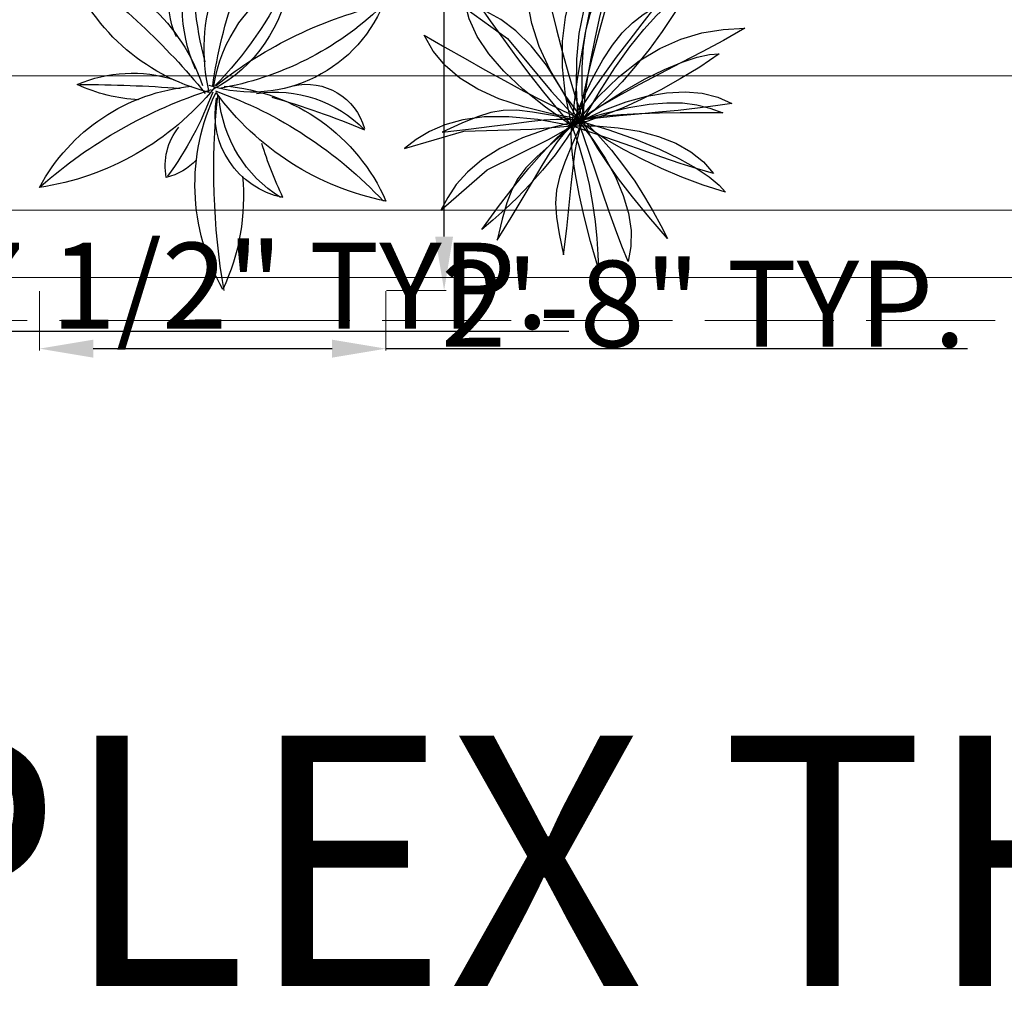
# Model space of a CAD drawing. Units: inches. Extents: x 351 to 1738, y -265 to 286.
# Tile 15 of 38: x 1176 to 1268, y -265 to -175. Entities that reach past the tile are written whole.
import ezdxf

# ---------------------------------------------------------------- set-up
doc = ezdxf.new("R2010")
doc.units = ezdxf.units.IN
doc.header["$MEASUREMENT"] = 0
doc.linetypes.add('ACAD_ISO02W100', pattern=[15, 12, -3])
for name, color, linetype, lineweight in [('A-ANNO-DIMS', 2, 'Continuous', 18), ('A-ANNO-TITL', 7, 'Continuous', 35), ('A-FLOR-OVHD', 1, 'ACAD_ISO02W100', 18), ('A-FLOR-PATT', 9, 'Continuous', 9)]:
    doc.layers.add(name, color=color, linetype=linetype, lineweight=lineweight)
for name, color, linetype in [('CAY', 94, 'Continuous'), ('CHITIET', 144, 'Continuous'), ('DIENHOA', 3, 'Continuous'), ('netmanh', 9, 'Continuous'), ('VATDUNG', 9, 'Continuous')]:
    doc.layers.add(name, color=color, linetype=linetype)
doc.styles.add('Annotative', font='arial.ttf')
doc.styles.get("Standard").update_dxf_attribs({"font": 'arial.ttf'})
doc.dimstyles.get("Standard").update_dxf_attribs({"dimtxt": 8, "dimasz": 5, "dimexe": 0.18, "dimexo": 0.0625, "dimgap": 0.09, "dimtad": 1, "dimtoh": 1, "dimzin": 0, "dimdsep": 46, "dimlunit": 4, "dimtxsty": 'Standard', "dimcen": 0, "dimclre": 256, "dimadec": 0, "dimazin": 0, "dimtfac": 1, "dimtofl": 0, "dimtmove": 0, "dimatfit": 3, "dimfxl": 1, "dimtolj": 1, "dimtzin": 0, "dimlwe": -1, "dimarcsym": 0})

# ---------------------------------------------------------------- blocks, each defined once
blk = doc.blocks.new('Cay03_mb')
at = {"layer": 'DIENHOA'}
for p, q in [((118.6, 555.3), (166.2, 599.1)), ((166.2, 599.1), (142.2, 519.4)), ((79.5, 503.7), (118.6, 555.3)), ((142.2, 519.4), (119, 441.7)), ((48.6, 443.6), (79.5, 503.7)), ((25.5, 374.3), (48.6, 443.6)), ((119, 441.7), (96.7, 365.6)), ((-365.2, 390.3), (-414.4, 402.8)), ((-414.4, 402.8), (-240.2, 277.8)), ((-314.9, 371.3), (-365.2, 390.3)), ((-263.5, 343.5), (-314.9, 371.3)), ((-211.2, 304.6), (-263.5, 343.5)), ((9.9, 295.3), (25.5, 374.3)), ((96.7, 365.6), (75.6, 290.6)), ((436.8, 297.2), (511, 309.6)), ((511, 309.6), (585.9, 313.5)), ((585.9, 313.5), (511.8, 271.4)), ((-240.2, 277.8), (-88.4, 94.9)), ((-158, 252.3), (-211.2, 304.6)), ((1.6, 205.7), (9.9, 295.3)), ((75.6, 290.6), (55.7, 216.3)), ((290.6, 243.2), (363.4, 275.4)), ((363.4, 275.4), (436.8, 297.2)), ((-104.2, 184.4), (-158, 252.3)), ((218.5, 199.8), (290.6, 243.2)), ((511.8, 271.4), (437.6, 231.5)), ((55.7, 216.3), (37.3, 142.1)), ((437.6, 231.5), (363.7, 192.9)), ((-49.6, 98.5), (-104.2, 184.4)), ((0.2, 104.9), (1.6, 205.7)), ((147, 144.1), (218.5, 199.8)), ((363.7, 192.9), (290.2, 154.9)), ((37.3, 142.1), (20.5, 67.6)), ((75.9, 75.2), (147, 144.1)), ((290.2, 154.9), (217.4, 116.6)), ((5.4, -7.8), (0.2, 104.9)), ((217.4, 116.6), (145.5, 77.3)), ((-88.4, 94.9), (5.4, -7.8)), ((5.4, -7.8), (-49.6, 98.5)), ((5.4, -7.8), (75.9, 75.2)), ((145.5, 77.3), (74.7, 36.1)), ((20.5, 67.6), (5.4, -7.8)), ((74.7, 36.1), (5.4, -7.8)), ((100.3, 18.4), (182.2, 37.2)), ((182.2, 37.2), (253, 48.9)), ((253, 48.9), (314.6, 54.1)), ((314.6, 54.1), (369.2, 53.3)), ((369.2, 53.3), (418.6, 46.8)), ((418.6, 46.8), (464.9, 35.2)), ((464.9, 35.2), (510, 19)), ((-345, 5.4), (-399.6, -17.1)), ((-298.6, 20.1), (-345, 5.4)), ((-254.7, 27.4), (-298.6, 20.1)), ((-208, 27.8), (-254.7, 27.4)), ((-152.7, 21.7), (-208, 27.8)), ((-83.4, 9.7), (-152.7, 21.7)), ((5.4, -7.8), (-83.4, 9.7)), ((5.4, -7.8), (100.3, 18.4)), ((46.3, 0.9), (5.4, -7.8)), ((96.7, 7.5), (46.3, 0.9)), ((155, 12.2), (96.7, 7.5)), ((219.6, 15.4), (155, 12.2)), ((289, 17.4), (219.6, 15.4)), ((361.6, 18.5), (289, 17.4)), ((435.8, 18.9), (361.6, 18.5)), ((510, 19), (435.8, 18.9)), ((-399.6, -17.1), (-468, -47.9)), ((-375.6, -37.8), (-295.3, -27.9)), ((-295.3, -27.9), (-225.8, -18.9)), ((-225.8, -18.9), (-165.8, -11.3)), ((-165.8, -11.3), (-114, -5.7)), ((-114, -5.7), (-69, -2.9)), ((-69, -2.9), (-29.6, -3.4)), ((-45.1, -46.3), (-16.5, -22.4)), ((5.4, -7.8), (-33.2, -69.5)), ((-29.6, -3.4), (5.4, -7.8)), ((-16.5, -22.4), (5.4, -7.8)), ((5.4, -7.8), (56.8, -73.3)), ((25.9, -64.4), (5.4, -7.8)), ((5.4, -7.8), (112.8, -40.3)), ((53.5, -41.6), (5.4, -7.8)), ((-468, -47.9), (-375.6, -37.8)), ((-79.8, -79.6), (-45.1, -46.3)), ((47, -125.9), (25.9, -64.4)), ((107, -75.7), (53.5, -41.6)), ((112.8, -40.3), (207.5, -73.8)), ((-120.2, -122.1), (-79.8, -79.6)), ((-33.2, -69.5), (-74.6, -127.3)), ((56.8, -73.3), (100.4, -139.1)), ((165.5, -109.6), (107, -75.7)), ((207.5, -73.8), (289.5, -107.6)), ((-165.9, -174.1), (-120.2, -122.1)), ((-74.6, -127.3), (-117.8, -181.1)), ((68.7, -190.6), (47, -125.9)), ((228.7, -142.8), (165.5, -109.6)), ((289.5, -107.6), (359.3, -141.1)), ((100.4, -139.1), (135.9, -204.3)), ((296, -174.7), (228.7, -142.8)), ((359.3, -141.1), (416.9, -173.5)), ((-216.3, -235.6), (-165.9, -174.1)), ((-117.8, -181.1), (-162.1, -230.9)), ((90.8, -256.6), (68.7, -190.6)), ((135.9, -204.3), (162.8, -268.3)), ((367.1, -204.8), (296, -174.7)), ((441.6, -232.7), (367.1, -204.8)), ((416.9, -173.5), (462.6, -204.2)), ((462.6, -204.2), (496.5, -232.5)), ((-271, -306.6), (-216.3, -235.6)), ((-162.1, -230.9), (-206.3, -276.5)), ((518.9, -257.7), (441.6, -232.7)), ((496.5, -232.5), (518.9, -257.7)), ((113.1, -322.2), (90.8, -256.6)), ((162.8, -268.3), (181, -330.4)), ((-329.5, -387.1), (-271, -306.6)), ((-206.3, -276.5), (-249.6, -317.8)), ((-249.6, -317.8), (-291, -354.7)), ((135.4, -385.6), (113.1, -322.2)), ((181, -330.4), (190, -390)), ((-291, -354.7), (-329.5, -387.1)), ((157.6, -445), (135.4, -385.6)), ((190, -390), (189.6, -446.3)), ((179.5, -498.7), (157.6, -445)), ((189.6, -446.3), (179.5, -498.7))]:
    blk.add_line(p, q, dxfattribs=at)
for points in [[(23.7, -5.4), (-41, 82.2), (-91.8, 167.1), (-129.7, 249.5), (-155.6, 329.6), (-170.2, 407.8), (-174.7, 484.2), (-169.8, 559.3), (-156.5, 633.1)], [(-156.5, 633.1), (-132.5, 551.3), (-110.5, 470), (-89.8, 389.2), (-69.6, 309), (-49, 229.4), (-27.1, 150.4), (-3.2, 72.1), (23.7, -5.4)], [(-16.4, -26.7), (-38.3, 80), (-48.9, 178.3), (-48.7, 269), (-38.5, 352.6), (-19.1, 429.7), (9, 501), (44.9, 567.1), (87.9, 628.5)], [(87.9, 628.5), (75.5, 544.2), (61.3, 461.2), (46.1, 379.1), (30.8, 297.8), (16.1, 216.9), (2.9, 136), (-8.3, 54.9), (-16.4, -26.7)], [(23.7, -5.4), (19.8, 93), (20.3, 177), (25, 248.5), (34, 309.8), (47.3, 362.7), (64.9, 409.3), (86.8, 451.7), (112.9, 491.9)], [(112.9, 491.9), (96, 419.7), (79.5, 347.4), (63.9, 276.5), (50, 208.4), (38.4, 144.8), (29.7, 86.9), (24.6, 36.3), (23.7, -5.4)], [(-395.6, 473.7), (-347.5, 405.6), (-300.6, 339.5), (-254.3, 275.1), (-208.3, 212.3), (-161.9, 150.9), (-114.8, 90.7), (-66.5, 31.6), (-16.4, -26.7)], [(-16.4, -26.7), (-108.3, 38.6), (-186.9, 101.7), (-252.4, 163.5), (-305.1, 224.4), (-345.4, 285.2), (-373.7, 346.6), (-390.4, 409.2), (-395.6, 473.7)], [(384.3, 437.5), (342.2, 367.8), (298.1, 301.7), (252.6, 239.4), (206.1, 181.1), (159.4, 127.2), (113, 78), (67.6, 33.6), (23.7, -5.4)], [(23.7, -5.4), (79.9, 91.7), (134.1, 176.2), (185.8, 248.4), (234.3, 308.7), (279, 357.3), (319.3, 394.8), (354.6, 421.4), (384.3, 437.5)], [(273.2, 387.3), (227.6, 328.8), (182.3, 270.1), (138.4, 212.3), (97.2, 156.4), (60, 103.4), (27.8, 54.6), (1.9, 10.8), (-16.4, -26.7)], [(-16.4, -26.7), (21.4, 64.2), (57, 140.3), (91.4, 203.3), (125.2, 255.1), (159.5, 297.5), (195, 332.5), (232.7, 361.8), (273.2, 387.3)], [(-530.5, 289.7), (-458.3, 248.1), (-387.9, 207.8), (-318.9, 168.7), (-250.8, 131.1), (-182.9, 94.8), (-114.9, 59.9), (-46.2, 26.5), (23.7, -5.4)], [(23.7, -5.4), (-87.2, 15.2), (-185, 39.6), (-270.3, 68.2), (-343.7, 101.4), (-405.9, 139.7), (-457.3, 183.5), (-498.7, 233.4), (-530.5, 289.7)], [(496.7, 224), (429.4, 178.4), (361.6, 136.9), (294.1, 99.5), (227.5, 66.1), (162.4, 36.7), (99.7, 11.5), (39.8, -9.7), (-16.4, -26.7)], [(-16.4, -26.7), (75.4, 37.9), (160.1, 91.8), (237.3, 135.7), (306.6, 170), (367.6, 195.4), (419.9, 212.5), (463.1, 221.9), (496.7, 224)], [(23.7, -5.4), (99.3, 29.7), (173.2, 57.1), (244.8, 76.7), (313.3, 88.3), (377.9, 91.8), (437.9, 87), (492.7, 73.8), (541.4, 52)], [(541.4, 52), (484.1, 42.9), (421.2, 34.8), (354.4, 27.6), (285.4, 20.9), (216.1, 14.5), (148.2, 8.1), (83.5, 1.6), (23.7, -5.4)], [(-16.4, -26.7), (-134, -4.7), (-235.3, 5.3), (-322, 4.7), (-395.9, -5), (-458.7, -22.3), (-512.3, -45.7), (-558.2, -73.6), (-598.4, -104.7)], [(-598.4, -104.7), (-392.7, -44.4), (-155, -37.4), (-16.4, -26.7)], [(-471.9, -320.3), (-310.5, -179.3), (-97.7, -73.3), (23.7, -5.4)], [(23.7, -5.4), (-92.3, -34.8), (-188.4, -68.2), (-266.9, -105.1), (-329.9, -144.9), (-379.7, -187), (-418.5, -230.7), (-448.5, -275.3), (-471.9, -320.3)], [(-276.2, -424.4), (-227.3, -345.4), (-185.7, -276.1), (-150, -215.7), (-119.1, -163.8), (-91.5, -119.5), (-66, -82.3), (-41.4, -51.6), (-16.4, -26.7)], [(-16.4, -26.7), (-84.9, -86), (-137, -133.1), (-175.8, -173), (-204.3, -210), (-225.5, -249.1), (-242.5, -294.7), (-258.4, -351.6), (-276.2, -424.4)], [(23.7, -5.4), (-13.6, -87.9), (-41.1, -152.6), (-59.6, -205), (-69.9, -250.7), (-72.8, -295), (-69.2, -343.6), (-59.7, -401.9), (-45.3, -475.5)], [(-45.3, -475.5), (-34.1, -383.2), (-25.4, -302.8), (-18.3, -233.1), (-12, -172.9), (-5.6, -121.2), (2, -76.8), (11.4, -38.5), (23.7, -5.4)], [(76.2, -524.2), (48.8, -428.5), (26.6, -341.7), (9.2, -264.1), (-3.6, -196.1), (-12.3, -138), (-17.1, -90.2), (-18.3, -53), (-16.4, -26.7)], [(-16.4, -26.7), (66.9, -26.6), (145.6, -32.7), (218.8, -44.9), (285.8, -63.1), (345.9, -87.1), (398.4, -116.6), (442.6, -151.6), (477.6, -191.8)], [(477.6, -191.8), (421.8, -176), (361.3, -156.9), (297.6, -135.5), (232.2, -112.6), (166.6, -89.4), (102.3, -66.6), (40.8, -45.4), (-16.4, -26.7)], [(-16.4, -26.7), (8.5, -95.1), (28.5, -163.3), (44.3, -230.6), (56.3, -296.1), (65, -359), (70.9, -418.5), (74.5, -473.9), (76.2, -524.2)], [(316.5, -418.1), (251.4, -342.8), (194.8, -273.3), (146.5, -210.2), (106.3, -153.8), (74.1, -104.7), (49.7, -63.4), (32.9, -30.1), (23.7, -5.4)], [(23.7, -5.4), (74.9, -57.1), (121.8, -110.6), (164.3, -165), (202.7, -219.4), (237, -272.9), (267.3, -324.5), (293.7, -373.2), (316.5, -418.1)]]:
    blk.add_lwpolyline(points, dxfattribs=at)
blk = doc.blocks.new('A$C5431134F')
at = {"layer": 'VATDUNG'}
for centre, radius, start, end in [((2160.8, 1662), 1245, 150.24114, 205.80899), ((5177, 1582.5), 4150.3, 170.23998, 186.11478), ((-65.9, 1738.8), 1267.2, 354.33263, 25.28039), ((193.1, 3473.3), 2507.8, 289.63177, 316.94159), ((2357.8, 162.2), 1629.1, 101.24862, 143.98987), ((1000.7, 2213.1), 1133.8, 274.40726, 336.44308), ((1532.8, 1250.1), 499, 101.42671, 190.98767), ((1828.1, 1082.8), 773.2, 121.90552, 175.18589), ((3715.1, 660.2), 2523.5, 154.68532, 162.45009), ((-246.7, 51.1), 1647.5, 39.15, 81.38898), ((1000.7, 2213.1), 1133.8, 208.0484, 264.64912), ((1859.5, 3770.4), 2797.6, 228.57445, 252.38422), ((1101.5, 1552.5), 361.2, 169.11662, 218.95559), ((667.9, 1279.8), 349.9, 42.83737, 76.97864), ((-929.9, 388.9), 2082.1, 20.51384, 36.02424), ((1386.4, 1856.4), 738.5, 261.63887, 315.62551), ((-169.9, 6392.7), 5465.7, 286.3355, 292.41502), ((1571.2, 1428.8), 356.3, 257.35568, 344.35325), ((624.5, 223.6), 940.4, 92.43736, 115.29557), ((1294.4, -49.6), 1206.1, 104.12842, 160.14677), ((-2233.8, 3749.8), 4146.2, 305.44636, 320.73815), ((2052.7, 864.5), 1083.3, 166.36026, 232.94739), ((1250.8, 281.5), 836.9, 19.43419, 107.43571), ((625, 349.3), 851.8, 6.50728, 62.3609), ((-65.9, 1738.8), 1267.2, 330.76974, 331.93672), ((-70, 1420), 1084.7, 282.24233, 341.73209), ((546.4, 1826.6), 819.5, 246.7315, 287.39709), ((248.9, 8461.8), 7388, 269.91003, 274.50199), ((3885.3, 1488.7), 2894, 188.09589, 210.72258), ((1889.6, 1210.8), 871.9, 188.55522, 241.3289), ((-527.8, -458.7), 2192.5, 24.75992, 44.64728), ((2594.9, 3037.7), 2500, 231.54163, 257.17636), ((754.1, -691.9), 1814.1, 46.14832, 80.37107), ((1738.9, 617.5), 897.6, 155.9893, 202.83996), ((2946.5, 414), 2039.9, 165.0604, 184.07375), ((1214.1, 597.8), 452.1, 154.5276, 228.0163), ((-246.7, 51.1), 1647.5, 358.22216, 17.85831)]:
    blk.add_arc(centre, radius, start, end, dxfattribs=at)
blk = doc.blocks.new('A$C5A8625A6')
at = {"layer": 'CHITIET', "ltscale": 50, "xscale": -0.49, "yscale": 0.49, "zscale": 0.49, "rotation": 180}
blk.add_blockref('A$C5431134F', (0, 1120.2), dxfattribs=at)
blk = doc.blocks.new('A$C18571848')
at = {"layer": 'netmanh', "xscale": 0.5393606399999998, "yscale": 0.5393606399999998, "zscale": 0.5393606399999998}
blk.add_blockref('A$C5A8625A6', (0, 0), dxfattribs=at)
blk = doc.blocks.new('*D36')
at = {"layer": 'A-ANNO-DIMS', "transparency": 16777216}
for p, q in [((1073.569, -199.341), (1073.569, -204.202)), ((1105.198, -199.341), (1105.198, -204.202))]:
    blk.add_line(p, q, dxfattribs=at)
at = {"layer": 'A-ANNO-DIMS', "color": 0, "lineweight": -2, "transparency": 16777216}
for p, q in [((1078.569, -204.022), (1100.198, -204.022)), ((1105.198, -204.022), (1227.071, -204.022))]:
    blk.add_line(p, q, dxfattribs=at)
at = {"layer": 'A-ANNO-DIMS', "color": 0, "transparency": 16777216}
for points in [[(1078.569, -203.189), (1078.569, -204.856), (1073.569, -204.022)], [(1100.198, -203.189), (1100.198, -204.856), (1105.198, -204.022)]]:
    blk.add_solid(points, dxfattribs=at)
at = {"layer": 'Defpoints', "color": 0, "transparency": 16777216}
for p in [(1073.569, -199.278), (1105.198, -199.278), (1105.198, -204.022)]:
    blk.add_point(p, dxfattribs=at)
at = {"layer": 'A-ANNO-DIMS', "color": 0, "transparency": 16777216, "insert": (1168.634, -199.796), "char_height": 8, "attachment_point": 5}
blk.add_mtext('\\A1;PLANT A 2\'-7 1/2" TYP.', dxfattribs=at)
blk = doc.blocks.new('*D38')
at = {"layer": 'A-ANNO-DIMS', "color": 0, "lineweight": -2, "transparency": 16777216}
for p, q in [((1215.465, -164.135), (1215.465, -159.135)), ((1215.465, -159.135), (1313.607, -159.135)), ((1215.465, -195.235), (1215.465, -169.135))]:
    blk.add_line(p, q, dxfattribs=at)
at = {"layer": 'A-ANNO-DIMS', "transparency": 16777216}
for p, q in [((1210.112, -164.135), (1215.645, -164.135)), ((1210.112, -200.235), (1215.645, -200.235))]:
    blk.add_line(p, q, dxfattribs=at)
at = {"layer": 'A-ANNO-DIMS', "color": 0, "transparency": 16777216}
for points in [[(1214.631, -169.135), (1216.298, -169.135), (1215.465, -164.135)], [(1214.631, -195.235), (1216.298, -195.235), (1215.465, -200.235)]]:
    blk.add_solid(points, dxfattribs=at)
at = {"layer": 'Defpoints', "color": 0, "transparency": 16777216}
for p in [(1210.05, -164.135), (1215.465, -164.135), (1210.05, -200.235)]:
    blk.add_point(p, dxfattribs=at)
at = {"layer": 'A-ANNO-DIMS', "color": 0, "transparency": 16777216, "insert": (1264.581, -154.958), "char_height": 8, "attachment_point": 5}
blk.add_mtext('\\A1;PLANT B 3\'-0" TYP.', dxfattribs=at)
blk = doc.blocks.new('*D39')
at = {"layer": 'A-ANNO-DIMS', "transparency": 16777216}
for p, q in [((1177.835, -200.297), (1177.835, -205.829)), ((1210.05, -200.297), (1210.05, -205.829))]:
    blk.add_line(p, q, dxfattribs=at)
at = {"layer": 'A-ANNO-DIMS', "color": 0, "lineweight": -2, "transparency": 16777216}
for p, q in [((1182.835, -205.649), (1205.05, -205.649)), ((1210.05, -205.649), (1264.13, -205.649))]:
    blk.add_line(p, q, dxfattribs=at)
at = {"layer": 'A-ANNO-DIMS', "color": 0, "transparency": 16777216}
for points in [[(1182.835, -204.816), (1182.835, -206.483), (1177.835, -205.649)], [(1205.05, -204.816), (1205.05, -206.483), (1210.05, -205.649)]]:
    blk.add_solid(points, dxfattribs=at)
at = {"layer": 'Defpoints', "color": 0, "transparency": 16777216}
for p in [(1177.835, -200.235), (1210.05, -200.235), (1210.05, -205.649)]:
    blk.add_point(p, dxfattribs=at)
at = {"layer": 'A-ANNO-DIMS', "color": 0, "transparency": 16777216, "insert": (1239.59, -201.475), "char_height": 8, "attachment_point": 5}
blk.add_mtext('\\A1;2\'-8" TYP.', dxfattribs=at)

msp = doc.modelspace()

# ---------------------------------------------------------------- hatches: boundary and pattern name
at = {"layer": 'A-FLOR-PATT', "transparency": 33554559}
h = msp.add_hatch(dxfattribs=at)
h.set_pattern_fill('ANSI32', color=256, scale=50, angle=135)
h.set_pattern_definition([(180, (1038.704, -199.037), (-2e-15, -18.75), []), (180, (1032.454, -192.787), (-2e-15, -18.75), [])])
h.paths.add_polyline_path([(1248.506, -102.915), (1236.559, -102.916), (1236.553, -56.864), (1112.704, -57.026), (1112.704, -57.037), (1103.704, -57.037), (1103.704, -45.037), (1103.704, 98.963), (1076.434, 98.963), (1076.549, -81.037), (1071.549, -81.037), (1043.704, -81.037), (1038.704, -81.037), (1038.704, -161.037), (1043.704, -161.037), (1043.704, -173.037), (1038.704, -173.037), (1038.704, -199.037), (1562.704, -199.037), (1562.704, -173.037), (1236.549, -173.037), (1236.549, -164.037), (1236.693, -164.037), (1236.676, -150.916), (1248.512, -150.915)])
h.paths.add_polyline_path([(1236.133, -134.078), (1247.348, -134.078), (1247.348, -122.929), (1236.133, -122.929)], flags=24)
h.paths.add_polyline_path([(1308.144, -185.548), (1321.66, -185.548), (1321.66, -174.4), (1308.144, -174.4)], flags=24)
h.paths.add_polyline_path([(1121.632, -122.88), (1179.647, -122.88), (1179.647, -112.309), (1121.632, -112.309)], flags=24)
h.paths.add_polyline_path([(1124.515, -112.593), (1177.986, -112.593), (1177.986, -101.056), (1124.515, -101.056)], flags=24)
h.paths.add_polyline_path([(1091.374, 23.58), (1104.89, 23.58), (1104.89, 34.728), (1091.374, 34.728)], flags=24)

# ---------------------------------------------------------------- linework, layer by layer
at = {"layer": 'A-FLOR-OVHD'}
for p, q in [((1562.704, -199.037), (1038.704, -199.037)), ((1566.704, -203.037), (1034.704, -203.037))]:
    msp.add_line(p, q, dxfattribs=at)

# ---------------------------------------------------------------- block references
at = {"layer": 'CAY'}
for name, p, xscale, yscale, zscale in [('A$C18571848', (1177.835, -200.235), 0.0597507335965459, 0.0597507335965459, 0.0597507335965459), ('Cay03_mb', (1227.774, -184.232), 0.0267074520028285, 0.0267074520028285, 0.0267074520028285)]:
    msp.add_blockref(name, p, dxfattribs=dict(at, xscale=xscale, yscale=yscale, zscale=zscale))

# ---------------------------------------------------------------- texts
at = {"layer": 'A-ANNO-TITL', "style": 'Annotative'}
msp.add_text('DUPLEX THIRD FLOOR', height=23.27476, dxfattribs=at).set_placement((1115.071, -264.89))

# ---------------------------------------------------------------- dimensions: what is measured, and where the dimension line sits
at = {"layer": 'A-ANNO-DIMS'}
dim = msp.add_linear_dim(base=(1215.465, -164.135), p1=(1210.05, -200.235), p2=(1210.05, -164.135), angle=90, text='PLANT B <> TYP.', dimstyle='Standard', override={"dimdec": 1, "dimlfac": 1, "dimrnd": 0, "dimzin": 1, "dimdsep": 46, "dimlunit": 4, "dimfrac": 2}, dxfattribs=at)
dim.commit()
dim.dimension.update_dxf_attribs({"geometry": '*D38', "text_midpoint": (1264.581, -154.958)})
for base, p1, p2, text, picture, middle in [((1105.198, -204.022), (1073.569, -199.278), (1105.198, -199.278), 'PLANT A <> TYP.', '*D36', (1168.634, -199.796)), ((1210.05, -205.649), (1177.835, -200.235), (1210.05, -200.235), '<> TYP.', '*D39', (1239.59, -201.475))]:
    dim = msp.add_linear_dim(base=base, p1=p1, p2=p2, text=text, dimstyle='Standard', override={"dimdec": 1, "dimlfac": 1, "dimrnd": 0, "dimzin": 1, "dimdsep": 46, "dimlunit": 4, "dimfrac": 2}, dxfattribs=at)
    dim.commit()
    dim.dimension.update_dxf_attribs({"geometry": picture, "text_midpoint": middle})

doc.saveas('drawing.dxf')
